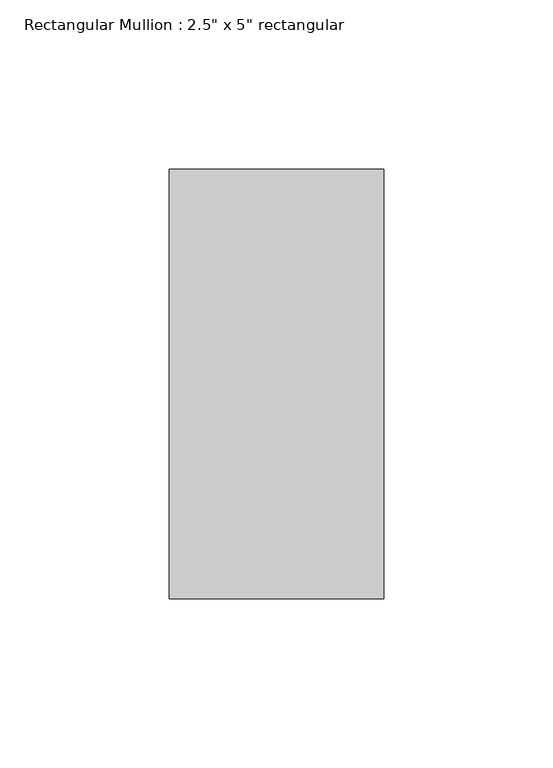
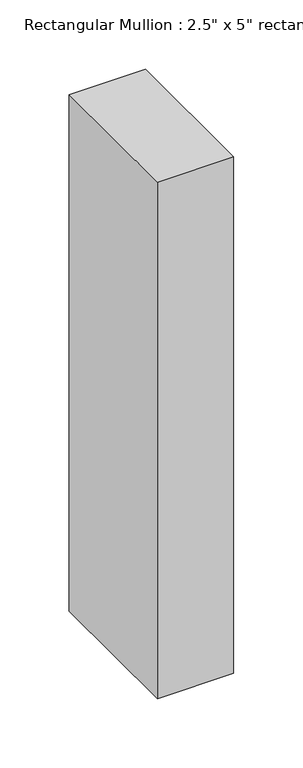
"""IFC4 building model written with IfcOpenShell, lengths in millimetres: member geometry."""

from ifc_helpers import new_model, si_unit, frame, origin, place, context, project, spatial, polyline, outline, extrude, source, transform, mapped, element, save


def member_9dbbeca1(model_context):
    return source(origin(), model_context, "Body", "SweptSolid", [
        extrude(outline(polyline([(0.0, 63.5), (0.0, -63.5), (-63.5, -63.5), (-63.5, 63.5), (0.0, 63.5)])), frame((0.0, 0.0, -454.025), z_axis=(0.0, 0.0, 1.0), x_axis=(1.0, 0.0, 0.0)), (0.0, 0.0, 1.0), 454.025),
    ])


if __name__ == "__main__":
    model = new_model("IFC4")
    model_context = context("Model", 3, world=origin())
    ifc_project = project(units=[si_unit("LENGTHUNIT", "METRE", prefix="MILLI")], contexts=[model_context])
    site = spatial("IfcSite", under=ifc_project)
    building = spatial("IfcBuilding", under=site)
    placement = place(None, origin())
    member_shape = member_9dbbeca1(model_context)
    element("IfcMember", 1, ObjectType="Rectangular Mullion : 2.5\" x 5\" rectangular", at=placement, inside=building, context=model_context, shape_type="MappedRepresentation", body=[
        mapped(member_shape, transform((0.0, 0.0, 0.0), x_axis=(1.0, 0.0, 0.0), y_axis=(0.0, 1.0, 0.0), z_axis=(0.0, 0.0, 1.0))),
    ])
    save(model, "model.ifc")

# Revit data of these elements
# Type "Rectangular Mullion : 2.5\" x 5\" rectangular"
#   built-in parameter 1007304 = 0.416667 (stored number, unit not read)
#   built-in parameter 1007301 = 0.104167 (stored number, unit not read)
#   built-in parameter 1007300 = 0.104167 (stored number, unit not read)
# Element 1 (IfcMember, "Rectangular Mullion : 2.5\" x 5\" rectangular")
#   Materials on its faces: "Aluminum"
# Materials
#   "Aluminum": class "Metal", colour RGB 247 247 247, transparency 0, Description = "Aluminum 6061", Cost = 0
